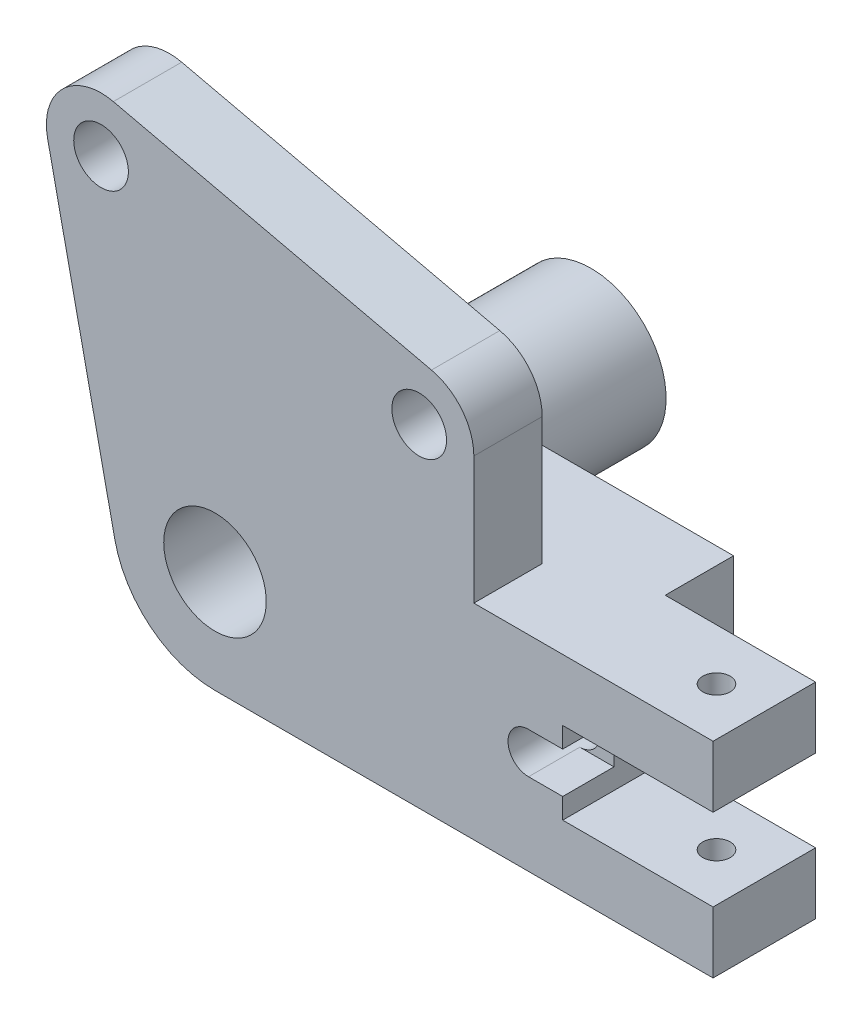
from build123d import *

# Parameters (mm, degrees)
BRACKET_PLATE_PROFILE_R     = 4
BRACKET_PLATE_DEPTH         = 25
FORK_SLOT_SKETCH_W          = 80.7543585
FORK_SLOT_SKETCH_H          = 21.257894267
FORK_SLOT_DEPTH             = 108.407683018
PIVOT_BOSS_SKETCH_R         = 11
PIVOT_BOSS_22_DEPTH         = 30
PIVOT_BORE_SKETCH_R         = 7.5
PIVOT_BORE_15_DEPTH         = 131.686611628
FORK_NOTCH_SKETCH_W         = 22
FORK_NOTCH_SKETCH_H         = 19.498267172
FORK_NOTCH_22X10_DEPTH      = 109.680312712
FORK_PIN_HOLE_SKETCH_R      = 2
FORK_PIN_HOLE_DEPTH         = 30
CLAMP_HOLE_SKETCH_R         = 3
CLAMP_HOLE_DEPTH            = 30
CLAMP_POCKET_SKETCH_W       = 7.221877003
CLAMP_POCKET_SKETCH_H       = 6
CLAMP_POCKET_7_5_DEEP_DEPTH = 7.5
HOLE_12_SKETCH_R            = 6
HOLE_12_DEPTH               = 10


with BuildPart() as part:
    # Bracket Plate Profile → Bracket Plate (new body)
    with BuildSketch(Plane.XY):
        with BuildLine():
            Line((0, 0), (-72.873763146, 0))
            ThreePointArc((-72.873763146, 0), (-82.303926322, 3.335008681), (-87.540799358, 11.857063669))
            Line((-87.540799358, 11.857063669), (-97.364307589, 57.700102084))
            ThreePointArc((-97.364307589, 57.700102084), (-95.154146662, 65.077436074), (-87.743012223, 67.171464359))
            Line((-87.743012223, 67.171464359), (-41.201123946, 56.431028603))
            ThreePointArc((-41.201123946, 56.431028603), (-36.739368705, 53.616310244), (-35, 48.635899037))
            Line((-35, 48.635899037), (-35, 30))
            Line((-35, 30), (0, 30))
            Line((0, 30), (0, 21))
            Line((0, 21), (-22, 21))
            Line((-22, 21), (-22, 9))
            Line((-22, 9), (0, 9))
            Line((0, 9), (0, 0))
        make_face()
        with Locations((-89.541888277, 59.376334794)):
            Circle(BRACKET_PLATE_PROFILE_R, mode=Mode.SUBTRACT)
        with Locations((-43, 48.635899037)):
            Circle(BRACKET_PLATE_PROFILE_R, mode=Mode.SUBTRACT)
    extrude(amount=BRACKET_PLATE_DEPTH)

    # Fork Slot Sketch → Fork Slot (cut, through all)
    with BuildSketch(Plane(origin=(0, 30, 0), x_dir=(1, 0, 0), z_dir=(0, 1, 0))):
        with Locations((-75.37717925, -4.371052867)):
            Rectangle(FORK_SLOT_SKETCH_W, FORK_SLOT_SKETCH_H)
    extrude(amount=FORK_SLOT_DEPTH, mode=Mode.SUBTRACT)

    # Pivot Boss Sketch → Pivot Boss Ø22 (add)
    with BuildSketch(Plane(origin=(0, 0, 0), x_dir=(-1, 0, 0), z_dir=(0, 0, -1))):
        with Locations((72.873763146, 15)):
            Circle(PIVOT_BOSS_SKETCH_R)
    extrude(amount=PIVOT_BOSS_22_DEPTH)

    # Pivot Bore Sketch → Pivot Bore Ø15 (cut, through all)
    with BuildSketch(Plane(origin=(0, 0, -30), x_dir=(-1, 0, 0), z_dir=(0, 0, -1))):
        with Locations((72.873763146, 15)):
            Circle(PIVOT_BORE_SKETCH_R)
    extrude(amount=-PIVOT_BORE_15_DEPTH, mode=Mode.SUBTRACT)

    # Fork Notch Sketch → Fork Notch 22x10 (cut, through all)
    with BuildSketch(Plane(origin=(0, 30, 0), x_dir=(1, 0, 0), z_dir=(0, 1, 0))):
        with Locations((-11, -0.250866414)):
            Rectangle(FORK_NOTCH_SKETCH_W, FORK_NOTCH_SKETCH_H)
    extrude(amount=-FORK_NOTCH_22X10_DEPTH, mode=Mode.SUBTRACT)

    # Fork Pin Hole Sketch → Fork Pin Hole (cut)
    with BuildSketch(Plane(origin=(0, 30, 0), x_dir=(1, 0, 0), z_dir=(0, 1, 0))):
        with Locations(Location((-7, -17.5, 0), (0, 0, 180))):
            Circle(FORK_PIN_HOLE_SKETCH_R)
    extrude(amount=-FORK_PIN_HOLE_DEPTH, mode=Mode.SUBTRACT)

    # Clamp Hole Sketch → Clamp Hole (cut)
    with BuildSketch(Plane.XY.offset(25)):
        with Locations((-27, 15)):
            Circle(CLAMP_HOLE_SKETCH_R)
    extrude(amount=-CLAMP_HOLE_DEPTH, mode=Mode.SUBTRACT)

    # Clamp Pocket Sketch → Clamp Pocket 7.5 Deep (cut)
    with BuildSketch(Plane.XY.offset(25)):
        with Locations((-23.389061498, 15)):
            Rectangle(CLAMP_POCKET_SKETCH_W, CLAMP_POCKET_SKETCH_H)
    extrude(amount=-CLAMP_POCKET_7_5_DEEP_DEPTH, mode=Mode.SUBTRACT)

    # Hole Ø12 Sketch → Hole Ø12 (cut)
    with BuildSketch(Plane(origin=(0, 0, 0), x_dir=(-1, 0, 0), z_dir=(0, 0, -1))):
        with Locations((27, 15)):
            Circle(HOLE_12_SKETCH_R)
    extrude(amount=-HOLE_12_DEPTH, mode=Mode.SUBTRACT)


solid = part.part
